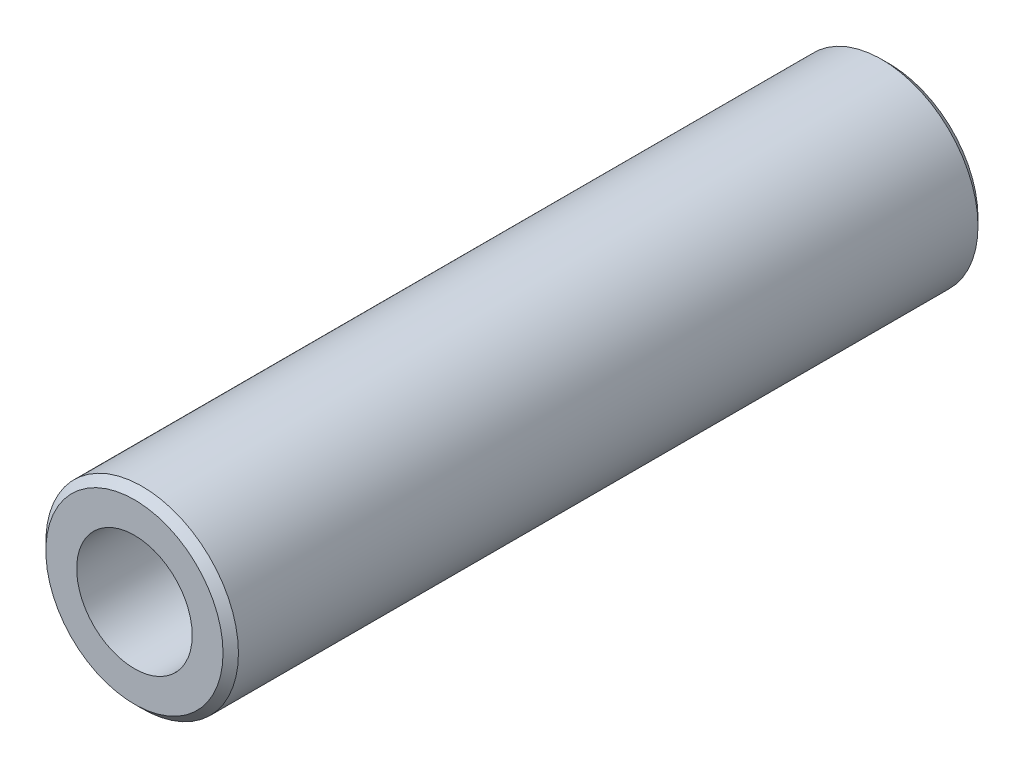
from build123d import *

# Parameters (mm, degrees)
PIN_OD_PROFILE_12_5_R        = 6.25
PIN_OD_PROFILE_12_5_R_2      = 3.75
PIN_TUBE_L49_WALL_2_5_DEPTH  = 24.5
PIN_EDGE_CHAMFER_0_5X45_SIZE = 0.5


with BuildPart() as part:
    # Pin OD Profile Ø12.5 → Pin Tube L49 Wall 2.5 (new, symmetric)
    with BuildSketch(Plane.XY):
        Circle(PIN_OD_PROFILE_12_5_R)
        Circle(PIN_OD_PROFILE_12_5_R_2, mode=Mode.SUBTRACT)
    extrude(amount=PIN_TUBE_L49_WALL_2_5_DEPTH, both=True)

    # Pin Edge Chamfer 0.5x45°
    pin_edge_chamfer_0_5x45_edges = [part.edges().sort_by_distance(p)[0] for p in [
        (-6.25, 0, -24.5),
        (-6.25, 0, 24.5),
    ]]
    chamfer(pin_edge_chamfer_0_5x45_edges, length=PIN_EDGE_CHAMFER_0_5X45_SIZE)


solid = part.part
